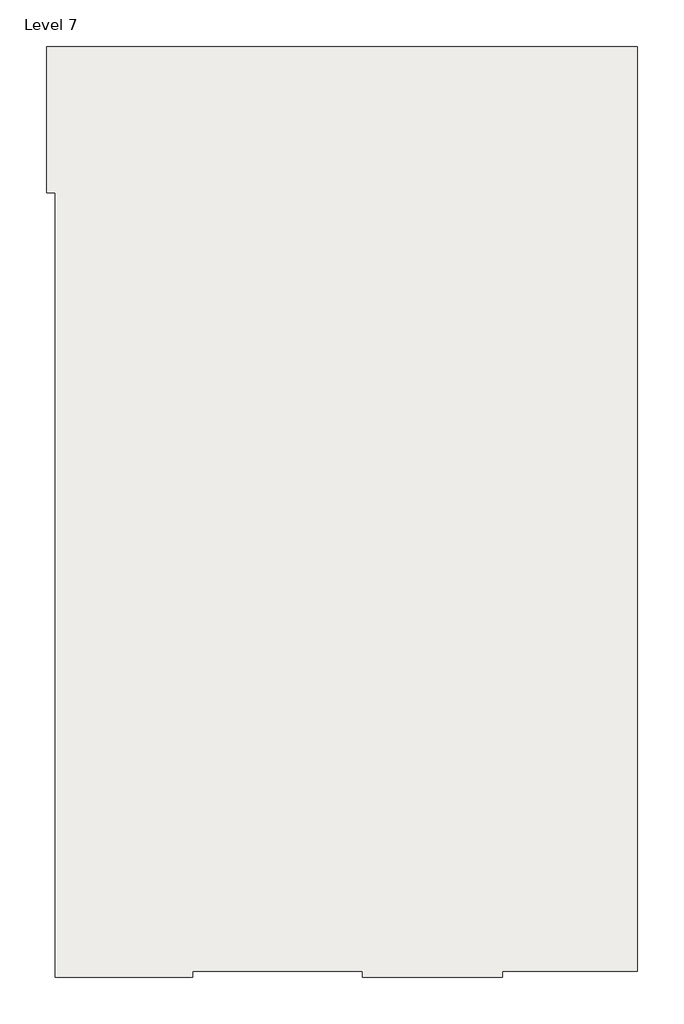
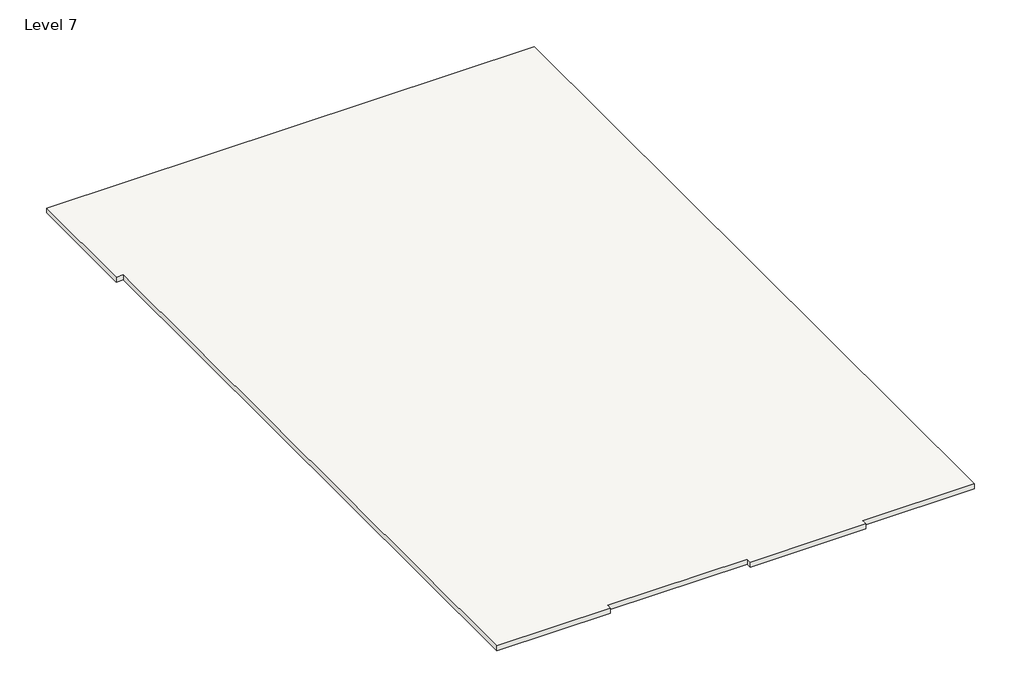
# One storey: 1 slab.
"""IFC4 building model written with IfcOpenShell, lengths in millimetres."""

from ifc_helpers import new_model, si_unit, frame, origin, place, context, project, spatial, polyline, outline, extrude, element, save

model = new_model("IFC4")

# Units and contexts
model_context = context("Model", 3, world=origin())
ifc_project = project(units=[si_unit("LENGTHUNIT", "METRE", prefix="MILLI")], contexts=[model_context])

# Site, building, storey
site = spatial("IfcSite", under=ifc_project)
building = spatial("IfcBuilding", under=site)
storey = spatial("IfcBuildingStorey", under=building, Name="Level 7", Elevation=13411.2)

# Slab
placement = place(None, origin())
element("IfcSlab", 1, ObjectType="6\" floor", at=placement, inside=storey, context=model_context, shape_type="SweptSolid", body=[
    extrude(outline(polyline([(5905.3208786, 11818.2189683), (5905.3208786, -10585.8779557), (2630.290751, -10585.8779557), (2630.290751, -10737.6531157), (-762.8431282, -10737.6531157), (-762.8431282, -10585.8779557), (-4874.3237038, -10585.8779557), (-4874.3237038, -10733.8493641), (-8210.307583, -10733.8493641), (-8210.307583, 8277.3011327), (-8419.607647, 8277.3011327), (-8419.607647, 11818.2189683), (5905.3208786, 11818.2189683)])), frame((0.0, 0.0, 13258.8), z_axis=(0.0, 0.0, 1.0), x_axis=(1.0, 0.0, 0.0)), (0.0, 0.0, 1.0), 152.4),
])

save(model, "model.ifc")

# Revit data of these elements
# Type "6\" floor"
#   Assembly Code = "B1010"
#   Function = 0
#   Layers, outside or top first: 0' - 6" no material (function 1)
# Element 1 (IfcSlab, "6\" floor")
#   Height Offset From Level = 0' - 0"
#   Phase Created = New Construction
#   Materials on its faces: "Default Floor"
# Materials
#   "Default Floor": colour RGB 128 128 128, transparency 0, Cost = 0
